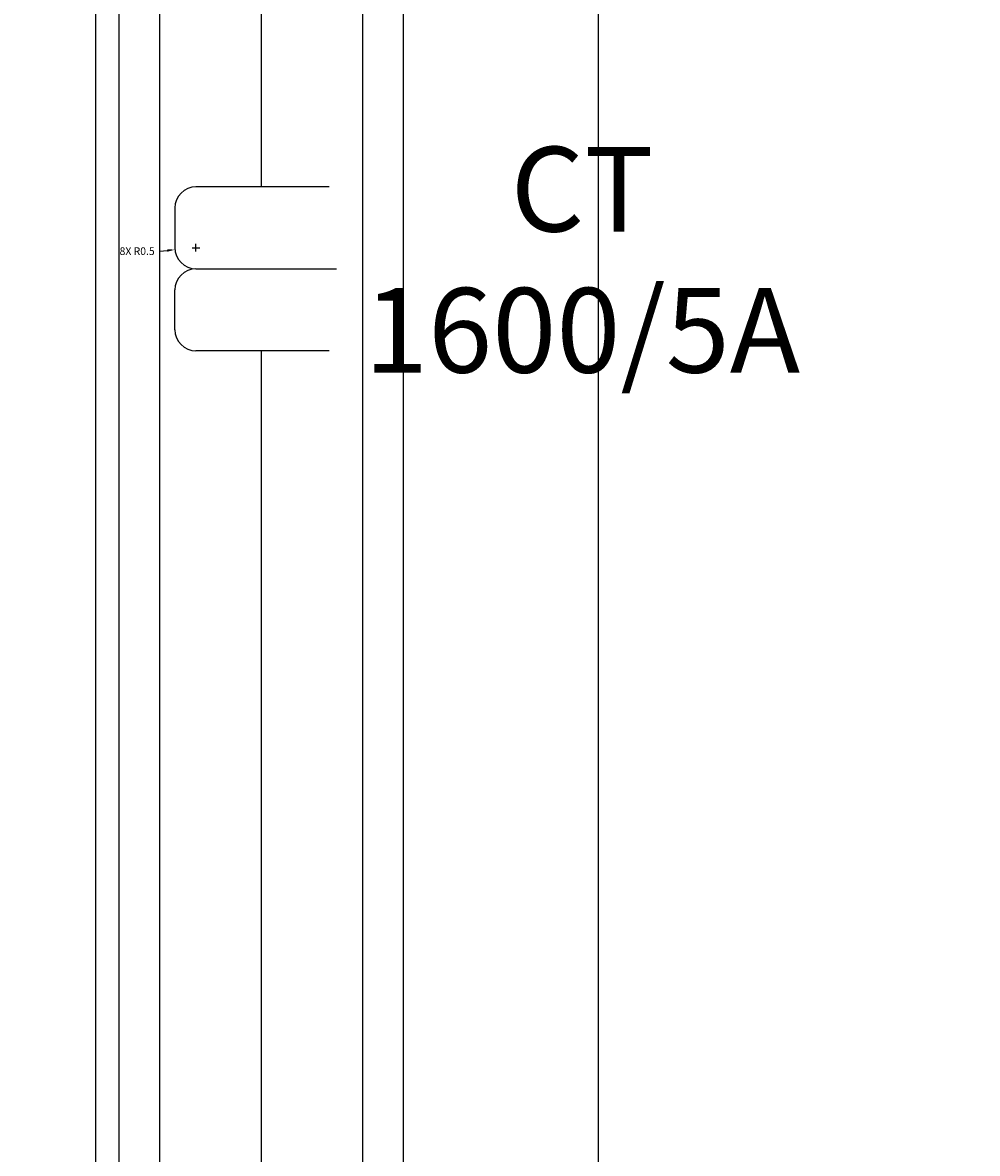
# Model space of a CAD drawing. Units: inches. Extents: x 412 to 584, y 208 to 437.
# Tile 11 of 28: x 494 to 516, y 262 to 288. Entities that reach past the tile are written whole.
import ezdxf

# ---------------------------------------------------------------- set-up
doc = ezdxf.new("R2010")
doc.units = ezdxf.units.IN
doc.header["$MEASUREMENT"] = 0
for name, color, linetype, lineweight in [('A-ANNO-DIMS', 2, 'Continuous', 18), ('E-ANNO-TEXT', 7, 'Continuous', 18), ('E-POWR-EQPM', 3, 'Continuous', 25)]:
    doc.layers.add(name, color=color, linetype=linetype, lineweight=lineweight)
doc.styles.get("Standard").update_dxf_attribs({"font": 'arial.ttf'})
doc.dimstyles.get("Standard").update_dxf_attribs({"dimtxt": 0.18, "dimasz": 0.18, "dimexe": 0.18, "dimexo": 0.0625, "dimgap": 0.09, "dimtad": 0, "dimtih": 1, "dimtoh": 1, "dimdec": 4, "dimzin": 0, "dimdsep": 46, "dimtxsty": 'Standard', "dimcen": 0.09, "dimadec": 0, "dimazin": 0, "dimtfac": 1, "dimtdec": 4, "dimtofl": 0, "dimtmove": 0, "dimatfit": 3, "dimfxl": 1, "dimtolj": 1, "dimtzin": 0, "dimarcsym": 0})

# ---------------------------------------------------------------- blocks, each defined once
blk = doc.blocks.new('CT-SYMBOL')
for p, q in [((3.642, 3.875), (0.5, 3.875)), ((0, 3.375), (0, 2.438)), ((0.5, 1.938), (3.819, 1.938)), ((0, 0.5), (0, 1.438)), ((3.642, 0), (0.5, 0))]:
    blk.add_line(p, q)
for centre, start, end in [((0.5, 3.375), 90, 180), ((0.5, 2.438), 180, 270), ((0.5, 1.438), 90, 180), ((0.5, 0.5), 180, 270)]:
    blk.add_arc(centre, 0.5, start, end)
blk = doc.blocks.new('*D17')
at = {"layer": 'A-ANNO-DIMS', "color": 0, "lineweight": -2, "transparency": 16777216}
for p, q in [((497.715, 426.185), (583.674, 426.185)), ((583.494, 426.005), (583.494, 323.031)), ((583.494, 219.693), (583.494, 322.667)), ((550.198, 219.513), (583.674, 219.513))]:
    blk.add_line(p, q, dxfattribs=at)
at = {"layer": 'A-ANNO-DIMS', "color": 0, "transparency": 16777216}
for points in [[(583.464, 426.005), (583.524, 426.005), (583.494, 426.185)], [(583.464, 219.693), (583.524, 219.693), (583.494, 219.513)]]:
    blk.add_solid(points, dxfattribs=at)
at = {"layer": 'Defpoints', "color": 0, "transparency": 16777216}
for p in [(497.652, 426.185), (550.135, 219.513), (583.494, 219.513)]:
    blk.add_point(p, dxfattribs=at)
at = {"layer": 'A-ANNO-DIMS', "color": 0, "transparency": 16777216, "insert": (583.494, 322.849), "char_height": 0.18, "attachment_point": 5}
blk.add_mtext('\\A1;206.67', dxfattribs=at)
blk = doc.blocks.new('*D28')
at = {"layer": 'A-ANNO-DIMS', "color": 0, "lineweight": -2, "transparency": 16777216}
for p, q in [((450.562, 256.635), (450.562, 437.465)), ((450.742, 437.285), (502.724, 437.285)), ((555.616, 437.285), (503.634, 437.285)), ((555.796, 256.635), (555.796, 437.465))]:
    blk.add_line(p, q, dxfattribs=at)
at = {"layer": 'A-ANNO-DIMS', "color": 0, "transparency": 16777216}
for points in [[(450.742, 437.315), (450.742, 437.255), (450.562, 437.285)], [(555.616, 437.315), (555.616, 437.255), (555.796, 437.285)]]:
    blk.add_solid(points, dxfattribs=at)
at = {"layer": 'Defpoints', "color": 0, "transparency": 16777216}
for p in [(555.796, 437.285), (450.562, 256.573), (555.796, 256.573)]:
    blk.add_point(p, dxfattribs=at)
at = {"layer": 'A-ANNO-DIMS', "color": 0, "transparency": 16777216, "insert": (503.179, 437.285), "char_height": 0.18, "attachment_point": 5}
blk.add_mtext('\\A1;105.23', dxfattribs=at)
blk = doc.blocks.new('*D29')
at = {"layer": 'A-ANNO-DIMS', "color": 0, "lineweight": -2, "transparency": 16777216}
for p, q in [((495.927, 378.924), (495.927, 208.233)), ((502.649, 378.924), (502.649, 208.233)), ((496.107, 208.413), (498.895, 208.413)), ((502.469, 208.413), (499.681, 208.413))]:
    blk.add_line(p, q, dxfattribs=at)
at = {"layer": 'A-ANNO-DIMS', "color": 0, "transparency": 16777216}
for points in [[(496.107, 208.443), (496.107, 208.383), (495.927, 208.413)], [(502.469, 208.443), (502.469, 208.383), (502.649, 208.413)]]:
    blk.add_solid(points, dxfattribs=at)
at = {"layer": 'Defpoints', "color": 0, "transparency": 16777216}
for p in [(495.927, 378.987), (502.649, 378.987), (502.649, 208.413)]:
    blk.add_point(p, dxfattribs=at)
at = {"layer": 'A-ANNO-DIMS', "color": 0, "transparency": 16777216, "insert": (499.288, 208.413), "char_height": 0.18, "attachment_point": 5}
blk.add_mtext('\\A1;6.722', dxfattribs=at)
blk = doc.blocks.new('*D31')
at = {"layer": 'A-ANNO-DIMS', "color": 0, "lineweight": -2, "transparency": 16777216}
for p, q in [((495.375, 405.385), (495.375, 208.233)), ((507.254, 405.385), (507.254, 208.233)), ((495.555, 208.413), (500.929, 208.413)), ((507.074, 208.413), (501.7, 208.413))]:
    blk.add_line(p, q, dxfattribs=at)
at = {"layer": 'A-ANNO-DIMS', "color": 0, "transparency": 16777216}
for points in [[(495.555, 208.443), (495.555, 208.383), (495.375, 208.413)], [(507.074, 208.443), (507.074, 208.383), (507.254, 208.413)]]:
    blk.add_solid(points, dxfattribs=at)
at = {"layer": 'Defpoints', "color": 0, "transparency": 16777216}
for p in [(495.375, 405.448), (507.254, 405.448), (507.254, 208.413)]:
    blk.add_point(p, dxfattribs=at)
at = {"layer": 'A-ANNO-DIMS', "color": 0, "transparency": 16777216, "insert": (501.314, 208.413), "char_height": 0.18, "attachment_point": 5}
blk.add_mtext('\\A1;11.88', dxfattribs=at)
blk = doc.blocks.new('*D39')
at = {"layer": 'A-ANNO-DIMS', "color": 0, "lineweight": -2, "transparency": 16777216}
for p, q in [((496.891, 346.914), (496.891, 208.233)), ((501.685, 346.914), (501.685, 208.233)), ((497.071, 208.413), (498.891, 208.413)), ((501.505, 208.413), (499.685, 208.413))]:
    blk.add_line(p, q, dxfattribs=at)
at = {"layer": 'A-ANNO-DIMS', "color": 0, "transparency": 16777216}
for points in [[(497.071, 208.443), (497.071, 208.383), (496.891, 208.413)], [(501.505, 208.443), (501.505, 208.383), (501.685, 208.413)]]:
    blk.add_solid(points, dxfattribs=at)
at = {"layer": 'Defpoints', "color": 0, "transparency": 16777216}
for p in [(496.891, 346.977), (501.685, 346.977), (501.685, 208.413)]:
    blk.add_point(p, dxfattribs=at)
at = {"layer": 'A-ANNO-DIMS', "color": 0, "transparency": 16777216, "insert": (499.288, 208.413), "char_height": 0.18, "attachment_point": 5}
blk.add_mtext('\\A1;4.794', dxfattribs=at)
blk = doc.blocks.new('*D51')
at = {"layer": 'A-ANNO-DIMS', "color": 0, "lineweight": -2, "transparency": 16777216}
for p, q in [((496.896, 282.971), (497.075, 282.988)), ((497.662, 283.053), (497.842, 283.053)), ((497.752, 282.963), (497.752, 283.143))]:
    blk.add_line(p, q, dxfattribs=at)
at = {"layer": 'A-ANNO-DIMS', "color": 0, "transparency": 16777216}
blk.add_solid([(497.072, 283.018), (497.078, 282.958), (497.254, 283.005)], dxfattribs=at)
at = {"layer": 'Defpoints', "color": 0, "transparency": 16777216}
for p in [(497.254, 283.005), (497.752, 283.053)]:
    blk.add_point(p, dxfattribs=at)
at = {"layer": 'A-ANNO-DIMS', "color": 0, "transparency": 16777216, "insert": (496.362, 282.971), "char_height": 0.18, "attachment_point": 5}
blk.add_mtext('\\A1;8X R0.5', dxfattribs=at)

msp = doc.modelspace()

# ---------------------------------------------------------------- linework, layer by layer
at = {"layer": 'E-POWR-EQPM'}
for p, q in [((499.2878, 299.3838), (499.2878, 284.4906)), ((499.2878, 280.6163), (499.2878, 276.6357)), ((499.2878, 276.6357), (499.2878, 256.9861))]:
    msp.add_line(p, q, dxfattribs=at)

# ---------------------------------------------------------------- block references
msp.add_blockref('CT-SYMBOL', (497.252, 280.6159), dxfattribs=at)

# ---------------------------------------------------------------- texts
at = {"layer": 'E-ANNO-TEXT', "insert": (498.5395, 285.4353), "char_height": 2, "attachment_point": 1}
msp.add_mtext_dynamic_manual_height_columns('\\pxqc;CT\\P1600/5A', width=16.663739, gutter_width=1, heights=[9.2096], dxfattribs=at)

# ---------------------------------------------------------------- dimensions: what is measured, and where the dimension line sits
at = {"layer": 'A-ANNO-DIMS'}
for base, p1, p2, override, picture, middle in [((555.7959, 437.2847), (450.562, 256.5729), (555.7959, 256.5729), {"dimdec": 2, "dimlfac": 1, "dimrnd": 0, "dimzin": 0, "dimdsep": 46, "dimlunit": 2}, '*D28', (503.1789, 437.2847)), ((507.2538, 208.4133), (495.3746, 405.448), (507.2538, 405.448), {"dimdec": 2, "dimlfac": 1, "dimrnd": 0, "dimzin": 0, "dimdsep": 46, "dimlunit": 2}, '*D31', (501.3142, 208.4133)), ((502.6489, 208.4133), (495.9268, 378.9867), (502.6489, 378.9867), {"dimdec": 3, "dimlfac": 1, "dimrnd": 0, "dimzin": 0, "dimdsep": 46, "dimlunit": 2}, '*D29', (499.2878, 208.4133)), ((501.6846, 208.4133), (496.891, 346.9765), (501.6846, 346.9765), {"dimdec": 3, "dimlfac": 1, "dimrnd": 0, "dimzin": 0, "dimdsep": 46, "dimlunit": 2}, '*D39', (499.2878, 208.4133))]:
    dim = msp.add_linear_dim(base=base, p1=p1, p2=p2, dimstyle='Standard', override=override, dxfattribs=at)
    dim.commit()
    dim.dimension.update_dxf_attribs({"geometry": picture, "text_midpoint": middle})
dim = msp.add_linear_dim(base=(583.4937, 219.5133), p1=(497.6523, 426.1847), p2=(550.1351, 219.5133), angle=90, dimstyle='Standard', override={"dimdec": 2, "dimlfac": 1, "dimrnd": 0, "dimzin": 0, "dimdsep": 46, "dimlunit": 2}, dxfattribs=at)
dim.commit()
dim.dimension.update_dxf_attribs({"geometry": '*D17', "text_midpoint": (583.4937, 322.849)})
dim = msp.add_radius_dim(center=(497.7518, 283.0534), mpoint=(497.2541, 283.0052), text='8X <>', dimstyle='Standard', override={"dimdec": 1, "dimlfac": 1, "dimrnd": 0, "dimzin": 0, "dimdsep": 46, "dimlunit": 2}, dxfattribs=at)
dim.commit()
dim.dimension.update_dxf_attribs({"geometry": '*D51', "text_midpoint": (496.3616, 282.9705)})

doc.saveas('drawing.dxf')
